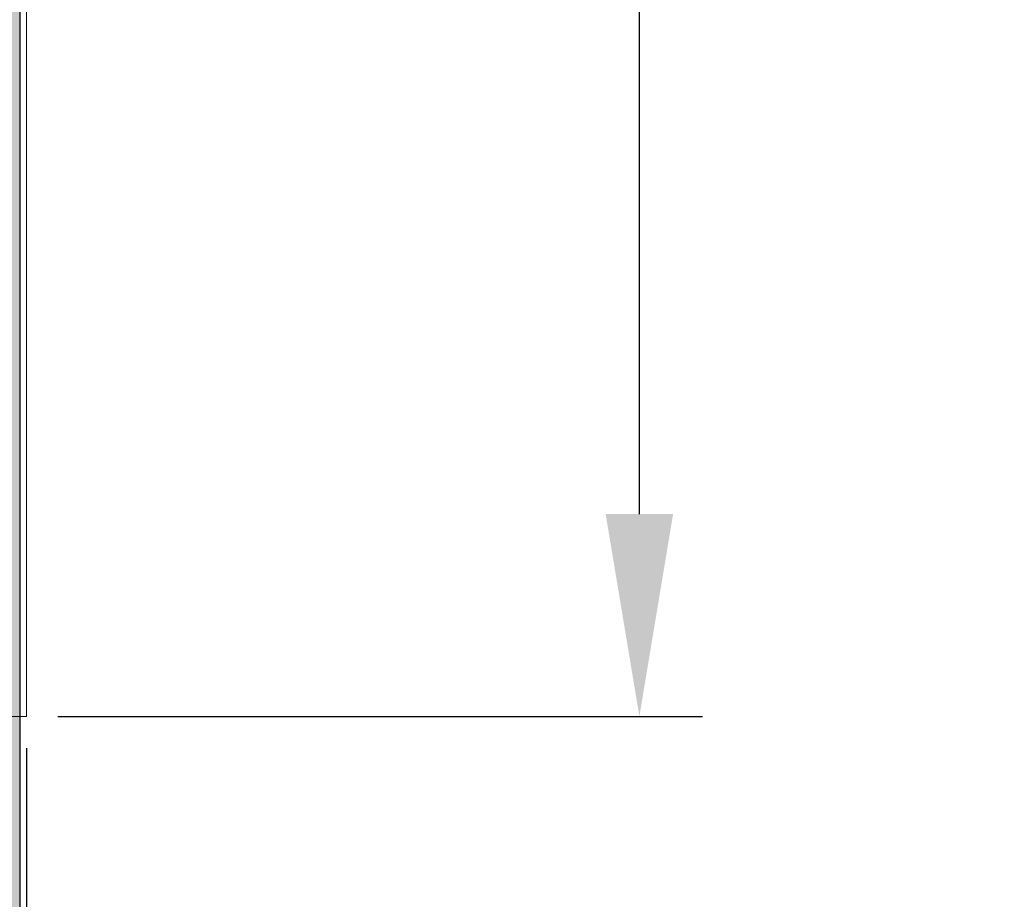
# Model space of a CAD drawing. Units: inches. Extents: x 2091 to 2899, y 967 to 2217.
# Tile 253 of 256: x 2212 to 2232, y 1149 to 1166. Entities that reach past the tile are written whole.
import ezdxf

# ---------------------------------------------------------------- set-up
doc = ezdxf.new("R2010")
doc.units = ezdxf.units.IN
doc.layers.add('A-ANNO-DIMS', color=2, linetype='Continuous', lineweight=18)
doc.layers.add('A-GLAZ', color=4, linetype='Continuous', lineweight=18)
doc.layers.add('A-WALL-PATT', color=141, linetype='Continuous', lineweight=13, true_color=0xadddf7)
doc.styles.get("Standard").update_dxf_attribs({"font": 'arial.ttf'})
doc.dimstyles.new('ISO-25', dxfattribs={"dimtxt": 4, "dimasz": 4, "dimexe": 1.25, "dimexo": 0.625, "dimtad": 1, "dimdec": 0, "dimlunit": 3, "dimtxsty": 'Standard', "dimcen": 2.5, "dimadec": 0, "dimazin": 0, "dimtfac": 1, "dimtdec": 0, "dimtmove": 0, "dimatfit": 3, "dimfxl": 1, "dimarcsym": 0})

# ---------------------------------------------------------------- blocks, each defined once
blk = doc.blocks.new('WIN-DOUBLE-LINE')
for p, q in [((9.16, 80.823), (9.16, 0)), ((9.16, 0), (0, 0))]:
    blk.add_line(p, q)
blk = doc.blocks.new('*D36')
at = {"layer": 'A-ANNO-DIMS', "color": 0, "lineweight": -2, "transparency": 16777216}
for p, q in [((2212.901, 1233.07), (2225.649, 1233.07)), ((2224.399, 1156.247), (2224.399, 1229.07)), ((2212.901, 1152.247), (2225.649, 1152.247))]:
    blk.add_line(p, q, dxfattribs=at)
at = {"layer": 'A-ANNO-DIMS', "color": 0, "transparency": 16777216}
for points in [[(2223.732, 1229.07), (2225.066, 1229.07), (2224.399, 1233.07)], [(2223.732, 1156.247), (2225.066, 1156.247), (2224.399, 1152.247)]]:
    blk.add_solid(points, dxfattribs=at)
at = {"layer": 'Defpoints', "color": 0, "transparency": 16777216}
for p in [(2212.276, 1233.07), (2224.399, 1233.07), (2212.276, 1152.247)]:
    blk.add_point(p, dxfattribs=at)
at = {"layer": 'A-ANNO-DIMS', "color": 0, "transparency": 16777216, "insert": (2221.705, 1192.659), "char_height": 4, "attachment_point": 5, "rotation": 90}
blk.add_mtext('WINDOW 6\'-9" TYP.', dxfattribs=at)
blk = doc.blocks.new('*D37')
at = {"layer": 'A-ANNO-DIMS', "color": 0, "lineweight": -2, "transparency": 16777216}
for p, q in [((2203.116, 1151.622), (2203.116, 1138.874)), ((2212.276, 1151.622), (2212.276, 1138.874)), ((2199.116, 1140.124), (2195.116, 1140.124)), ((2203.116, 1140.124), (2212.276, 1140.124)), ((2216.276, 1140.124), (2245.908, 1140.124))]:
    blk.add_line(p, q, dxfattribs=at)
at = {"layer": 'A-ANNO-DIMS', "color": 0, "transparency": 16777216}
for points in [[(2199.116, 1140.79), (2199.116, 1139.457), (2203.116, 1140.124)], [(2216.276, 1140.79), (2216.276, 1139.457), (2212.276, 1140.124)]]:
    blk.add_solid(points, dxfattribs=at)
at = {"layer": 'Defpoints', "color": 0, "transparency": 16777216}
for p in [(2203.116, 1152.247), (2212.276, 1152.247), (2212.276, 1140.124)]:
    blk.add_point(p, dxfattribs=at)
at = {"layer": 'A-ANNO-DIMS', "color": 0, "transparency": 16777216, "insert": (2233.092, 1142.791), "char_height": 4, "attachment_point": 5}
blk.add_mtext('0\'-9" TYP.', dxfattribs=at)
blk = doc.blocks.new('*D71')
at = {"layer": 'A-ANNO-DIMS', "color": 0, "lineweight": -2, "transparency": 16777216}
for p, q in [((2212.144, 1351.294), (2212.144, 969.464)), ((2452.144, 1351.294), (2452.144, 969.464)), ((2216.144, 970.714), (2448.144, 970.714))]:
    blk.add_line(p, q, dxfattribs=at)
at = {"layer": 'A-ANNO-DIMS', "color": 0, "transparency": 16777216}
for points in [[(2216.144, 971.381), (2216.144, 970.048), (2212.144, 970.714)], [(2448.144, 971.381), (2448.144, 970.048), (2452.144, 970.714)]]:
    blk.add_solid(points, dxfattribs=at)
at = {"layer": 'Defpoints', "color": 0, "transparency": 16777216}
for p in [(2212.144, 1351.919), (2452.144, 1351.919), (2452.144, 970.714)]:
    blk.add_point(p, dxfattribs=at)
at = {"layer": 'A-ANNO-DIMS', "color": 0, "transparency": 16777216, "insert": (2332.144, 973.382), "char_height": 4, "attachment_point": 5}
blk.add_mtext('20\'-0"', dxfattribs=at)
blk = doc.blocks.new('*D75')
at = {"layer": 'A-ANNO-DIMS', "color": 0, "lineweight": -2, "transparency": 16777216}
for p, q in [((2212.144, 1274.794), (2212.144, 969.464)), ((2308.144, 1274.794), (2308.144, 969.464)), ((2216.144, 970.714), (2304.144, 970.714))]:
    blk.add_line(p, q, dxfattribs=at)
at = {"layer": 'A-ANNO-DIMS', "color": 0, "transparency": 16777216}
for points in [[(2216.144, 971.381), (2216.144, 970.048), (2212.144, 970.714)], [(2304.144, 971.381), (2304.144, 970.048), (2308.144, 970.714)]]:
    blk.add_solid(points, dxfattribs=at)
at = {"layer": 'Defpoints', "color": 0, "transparency": 16777216}
for p in [(2212.144, 1275.419), (2308.144, 1275.419), (2308.144, 970.714)]:
    blk.add_point(p, dxfattribs=at)
at = {"layer": 'A-ANNO-DIMS', "color": 0, "transparency": 16777216, "insert": (2260.144, 973.382), "char_height": 4, "attachment_point": 5}
blk.add_mtext('8\'-0"', dxfattribs=at)
blk = doc.blocks.new('*D91')
at = {"layer": 'A-ANNO-DIMS', "color": 0, "lineweight": -2, "transparency": 16777216}
for p, q in [((2211.651, 1152.247), (2098.311, 1152.247)), ((2099.561, 1103.919), (2099.561, 1148.247)), ((2211.519, 1099.919), (2098.311, 1099.919))]:
    blk.add_line(p, q, dxfattribs=at)
at = {"layer": 'A-ANNO-DIMS', "color": 0, "transparency": 16777216}
for points in [[(2098.895, 1148.247), (2100.228, 1148.247), (2099.561, 1152.247)], [(2098.895, 1103.919), (2100.228, 1103.919), (2099.561, 1099.919)]]:
    blk.add_solid(points, dxfattribs=at)
at = {"layer": 'Defpoints', "color": 0, "transparency": 16777216}
for p in [(2099.561, 1152.247), (2212.276, 1152.247), (2212.144, 1099.919)]:
    blk.add_point(p, dxfattribs=at)
at = {"layer": 'A-ANNO-DIMS', "color": 0, "transparency": 16777216, "insert": (2096.868, 1126.083), "char_height": 4, "attachment_point": 5, "rotation": 90}
blk.add_mtext('4\'-4 1/2"', dxfattribs=at)

msp = doc.modelspace()

# ---------------------------------------------------------------- hatches: boundary and pattern name
at = {"layer": 'A-WALL-PATT'}
h = msp.add_hatch(color=256, dxfattribs=at)
h.dxf.hatch_style = 1
h.paths.add_polyline_path([(2803.144, 2050.919), (2203.144, 2050.919), (2203.144, 1090.919), (2803.144, 1090.919)])
h.paths.add_polyline_path([(2635.799, 1147.54), (2674.524, 1147.54, 0.376086), (2678.53, 1152.88), (2678.53, 1159.556, 0.333335), (2674.524, 1163.562), (2674.524, 1163.562), (2674.524, 1192.934), (2635.806, 1192.934), (2597.088, 1192.934), (2597.088, 1163.562, 0.333335), (2593.082, 1159.556), (2593.082, 1152.88, 0.376086), (2597.088, 1147.54)], flags=0)
h.paths.add_polyline_path([(2436.01, 1278.241, 0.000483), (2435.953, 1278.215, -0.001328), (2435.936, 1278.112, -0.001711), (2436.116, 1278.041, 0.002185)], flags=0)
h.paths.add_polyline_path([(2794.144, 1143.419), (2794.144, 1347.419), (2543.37, 1347.419), (2543.37, 1351.919), (2794.144, 1351.919), (2794.144, 1392.714), (2793.947, 1392.714), (2793.947, 1473.537), (2794.144, 1473.537), (2794.144, 1531.919), (2650.144, 1531.919), (2650.144, 1536.419), (2794.144, 1536.419), (2794.144, 1692.419), (2609.376, 1692.419), (2609.376, 1644.419), (2604.876, 1644.419), (2604.876, 1744.919), (2609.376, 1744.919), (2609.376, 1696.919), (2794.144, 1696.919), (2794.144, 1780.919), (2609.644, 1780.919), (2493.876, 1780.919), (2493.876, 1785.419), (2609.644, 1785.419), (2794.144, 1785.419), (2794.144, 1847.939), (2793.951, 1847.939), (2793.951, 1928.762), (2794.144, 1928.762), (2794.144, 1941.419), (2614.144, 1941.419), (2614.144, 1821.419), (2609.644, 1821.419), (2609.644, 1941.419), (2392.144, 1941.419), (2392.144, 1819.919), (2387.644, 1819.919), (2387.644, 1941.419), (2212.144, 1941.419), (2212.144, 1783.919), (2392.144, 1783.919), (2392.144, 1780.919), (2212.144, 1780.919), (2212.144, 1629.419), (2387.644, 1629.419), (2387.644, 1744.919), (2392.144, 1744.919), (2392.144, 1627.919), (2317.144, 1627.919), (2317.144, 1551.419), (2317.144, 1536.419), (2459.384, 1536.419), (2459.384, 1602.396), (2463.884, 1602.396), (2463.884, 1531.919), (2456.644, 1531.919), (2456.644, 1529.919), (2452.144, 1529.919), (2452.144, 1531.919), (2312.644, 1531.919), (2312.644, 1551.419), (2306.144, 1551.419), (2306.144, 1555.919), (2308.144, 1555.919), (2308.144, 1551.419), (2312.644, 1551.419), (2312.644, 1627.919), (2212.144, 1627.919), (2212.144, 1555.919), (2270.144, 1555.919), (2270.144, 1551.419), (2212.144, 1551.419), (2212.144, 1351.919), (2272.144, 1351.919), (2272.144, 1347.419), (2212.144, 1347.419), (2212.144, 1275.419), (2308.144, 1275.419), (2308.144, 1351.919), (2452.144, 1351.919), (2452.144, 1493.919), (2456.644, 1493.919), (2456.644, 1347.419), (2312.644, 1347.419), (2312.644, 1270.919), (2212.144, 1270.919), (2212.144, 1099.919), (2281.238, 1099.919), (2282.871, 1110.914), (2282.008, 1116.997), (2278.558, 1121.42), (2268.206, 1128.056), (2272.088, 1128.056), (2273.813, 1131.927), (2279.42, 1134.692), (2285.028, 1135.245), (2287.616, 1137.457), (2288.047, 1138.01), (2289.341, 1140.775), (2291.067, 1139.669), (2292.361, 1135.245), (2295.38, 1136.904), (2296.243, 1135.798), (2297.105, 1133.033), (2300.125, 1138.01), (2303.144, 1138.01), (2304.438, 1135.798), (2303.144, 1133.586), (2306.595, 1134.692), (2307.889, 1133.033), (2310.908, 1135.245), (2313.927, 1134.139), (2315.627, 1132.427), (2308.32, 1117.55), (2290.204, 1109.808), (2288.91, 1103.172), (2289.272, 1099.919), (2434.918, 1099.919), (2431.593, 1124.788), (2429.93, 1169.553), (2430.927, 1240.52), (2435.659, 1238.186), (2437.135, 1196.554), (2438.798, 1143.973), (2442.678, 1111.998), (2446.558, 1099.919), (2794.144, 1099.919), (2794.144, 1138.919), (2548.032, 1138.919), (2548.032, 1143.419), (2548.032, 1148.819), (2546.668, 1148.032), (2528.686, 1179.179, 0.256256), (2512.032, 1148.819), (2512.032, 1143.419), (2512.032, 1138.919), (2507.532, 1138.919), (2507.532, 1143.419), (2507.532, 1148.819, 0.256256), (2490.879, 1179.179), (2472.896, 1148.032), (2471.532, 1148.819), (2471.532, 1143.419), (2467.032, 1143.419), (2467.032, 1269.946, 0.039061), (2460.91, 1273.58), (2467.032, 1273.58), (2467.032, 1286.325, 0.014511), (2465.216, 1286.762), (2467.032, 1287.053), (2467.032, 1323.419), (2471.532, 1323.419), (2471.532, 1148.819), (2489.532, 1179.996), (2490.896, 1179.208), (2490.879, 1179.179, -0.256256), (2507.532, 1148.819), (2507.532, 1143.419), (2512.032, 1143.419), (2512.032, 1148.819, -0.256256), (2528.686, 1179.179), (2528.668, 1179.208), (2530.032, 1179.996), (2548.032, 1148.819), (2548.032, 1143.419)], flags=16)
h.paths.add_polyline_path([(2607.769, 1200.945), (2607.769, 1265.031), (2597.088, 1281.052), (2619.785, 1281.052), (2627.795, 1337.127), (2635.799, 1337.127), (2643.817, 1337.127), (2651.827, 1281.052), (2674.524, 1281.052), (2663.843, 1265.031), (2663.843, 1200.945), (2635.806, 1200.945)], flags=0)
edge = h.paths.add_edge_path(flags=0)
edge.add_ellipse((13303.896, 1272.999), major_axis=(-10595.313, 0), ratio=0.84230387, start_angle=0.6282372, end_angle=0.6465541, ccw=False)
edge.add_ellipse((2711.7, 1156.853), major_axis=(2.22, 0), ratio=0.842304, start_angle=111.5352, end_angle=180.6282, ccw=False)
edge.add_ellipse((13303.156, 1272.999), major_axis=(-10593.026, 0), ratio=0.84230387, start_angle=0.5282715, end_angle=0.6465541, ccw=False)
edge.add_line((2710.765, 1175.333), (2710.13, 1175.333))
edge.add_ellipse((2710.13, 1176.58), major_axis=(1.48, 0), ratio=0.842304, start_angle=180, end_angle=270, ccw=False)
edge.add_line((2708.65, 1176.58), (2708.65, 1200.783))
edge.add_ellipse((2710.13, 1200.783), major_axis=(1.48, 0), ratio=0.842304, start_angle=90, end_angle=180, ccw=False)
edge.add_line((2710.13, 1202.029), (2710.465, 1202.029))
edge.add_ellipse((13303.156, 1272.999), major_axis=(-10593.026, 0), ratio=0.84230387, start_angle=-0.0902291, end_angle=0.3838668, ccw=False)
edge.add_ellipse((2710.13, 1290.927), major_axis=(-1.48, 0), ratio=0.842304, start_angle=0, end_angle=90, ccw=False)
edge.add_line((2708.65, 1290.927), (2708.65, 1315.13))
edge.add_ellipse((2710.13, 1315.13), major_axis=(-1.48, 0), ratio=0.842304, start_angle=-90, end_angle=0, ccw=False)
edge.add_line((2710.13, 1316.377), (2710.706, 1316.377))
edge.add_ellipse((3238.402, 1296.29), major_axis=(528.234, 0), ratio=0.8423039, start_angle=176.34957, end_angle=177.82005, ccw=False)
edge.add_ellipse((2775.063, 1071.451), major_axis=(313.308, 0), ratio=0.8423039, start_angle=102.12597, end_angle=103.78053, ccw=False)
edge.add_ellipse((2775.063, 1078.306), major_axis=(-305.303, 0), ratio=0.8423039, start_angle=-79.79046, end_angle=-77.55537, ccw=False)
edge.add_ellipse((2695.142, 1541.975), major_axis=(-250.96, 0), ratio=0.8423039, start_angle=99.25657, end_angle=102.55493)
edge.add_line((2741.41, 1334.214), (2747.133, 1337.378))
edge.add_ellipse((2747.539, 1336.857), major_axis=(-0.74, 0), ratio=0.842304, start_angle=270, end_angle=307.9331, ccw=False)
edge.add_ellipse((2747.539, 1336.857), major_axis=(-0.74, 0), ratio=0.842304, start_angle=232.0669, end_angle=270, ccw=False)
edge.add_line((2747.945, 1337.378), (2753.667, 1334.214))
edge.add_ellipse((2799.935, 1541.975), major_axis=(250.96, 0), ratio=0.8423039, start_angle=257.44507, end_angle=260.74343)
edge.add_ellipse((2720.014, 1078.306), major_axis=(305.303, 0), ratio=0.8423039, start_angle=77.55537, end_angle=79.79046, ccw=False)
edge.add_ellipse((2720.014, 1071.451), major_axis=(-313.308, 0), ratio=0.8423039, start_angle=256.21947, end_angle=257.87403, ccw=False)
edge.add_ellipse((2256.676, 1296.29), major_axis=(-528.234, 0), ratio=0.8423039, start_angle=182.17995, end_angle=183.65043, ccw=False)
edge.add_line((2784.371, 1316.377), (2784.947, 1316.377))
edge.add_ellipse((2784.947, 1315.13), major_axis=(1.48, 0), ratio=0.842304, start_angle=0, end_angle=90, ccw=False)
edge.add_line((2786.427, 1315.13), (2786.427, 1290.927))
edge.add_ellipse((2784.947, 1290.927), major_axis=(1.48, 0), ratio=0.842304, start_angle=270, end_angle=360, ccw=False)
edge.add_ellipse((-7808.079, 1272.999), major_axis=(10593.026, 0), ratio=0.84230387, start_angle=-0.3838668, end_angle=0.0902291, ccw=False)
edge.add_line((2784.612, 1202.029), (2784.947, 1202.029))
edge.add_ellipse((2784.947, 1200.783), major_axis=(1.48, 0), ratio=0.842304, start_angle=0, end_angle=90, ccw=False)
edge.add_line((2786.427, 1200.783), (2786.427, 1176.58))
edge.add_ellipse((2784.947, 1176.58), major_axis=(-1.48, 0), ratio=0.842304, start_angle=90, end_angle=180, ccw=False)
edge.add_line((2784.947, 1175.333), (2784.313, 1175.333))
edge.add_ellipse((-7808.079, 1272.999), major_axis=(10593.026, 0), ratio=0.84230387, start_angle=-0.6186432, end_angle=-0.5282715, ccw=False)
edge.add_ellipse((2783.377, 1156.853), major_axis=(-2.22, 0), ratio=0.842304, start_angle=179.3718, end_angle=248.4648, ccw=False)
edge.add_ellipse((-7808.819, 1272.999), major_axis=(-10595.313, 0), ratio=0.842303866, start_angle=179.3534459, end_angle=179.3717628, ccw=False)
edge.add_ellipse((2780.297, 1153.501), major_axis=(-5.246, 0), ratio=0.842304, start_angle=90, end_angle=179.3534, ccw=False)
edge.add_line((2780.297, 1149.082), (2714.78, 1149.082))
edge.add_ellipse((2714.78, 1153.501), major_axis=(5.246, 0), ratio=0.842304, start_angle=180.6466, end_angle=270, ccw=False)
edge = h.paths.add_edge_path(flags=0)
edge.add_line((2718.187, 1151.008), (2718.187, 1170.472))
edge.add_ellipse((2721.147, 1170.472), major_axis=(-2.96, 0), ratio=0.842304, start_angle=-90, end_angle=0, ccw=False)
edge.add_line((2721.147, 1172.965), (2773.93, 1172.965))
edge.add_ellipse((2773.93, 1170.472), major_axis=(-2.96, 0), ratio=0.842304, start_angle=180, end_angle=270, ccw=False)
edge.add_line((2776.89, 1170.472), (2776.89, 1151.008))
edge.add_line((2776.89, 1151.008), (2718.187, 1151.008))
edge = h.paths.add_edge_path(flags=0)
edge.add_line((2718.187, 1180.234), (2718.187, 1199.058))
edge.add_ellipse((2747.539, 1320.399), major_axis=(147.018, 0), ratio=0.8423039, start_angle=256.40187, end_angle=283.59813)
edge.add_line((2776.89, 1199.058), (2776.89, 1180.234))
edge.add_ellipse((2747.539, 1301.575), major_axis=(147.018, 0), ratio=0.8423039, start_angle=256.40187, end_angle=283.59813, ccw=False)
edge = h.paths.add_edge_path(flags=0)
edge.add_ellipse((13303.156, 1272.999), major_axis=(-10591.546, 0), ratio=0.84230387, start_angle=0.0555943, end_angle=0.3777642, ccw=False)
edge.add_line((2711.617, 1262.722), (2715.667, 1249.495))
edge.add_ellipse((6413.892, 1241.692), major_axis=(-3698.236, 0), ratio=0.84230387, start_angle=-0.120897, end_angle=0.364076)
edge.add_line((2715.761, 1218.192), (2711.934, 1203.167))
edge = h.paths.add_edge_path(flags=0)
edge.add_line((2718.187, 1251.075), (2716.002, 1267.45))
edge.add_ellipse((2742.151, 1202.19), major_axis=(81.773, 0), ratio=0.842304, start_angle=94.27742, end_angle=111.83495, ccw=False)
edge.add_line((2737.01, 1270.931), (2758.067, 1270.931))
edge.add_ellipse((2752.926, 1202.19), major_axis=(81.773, 0), ratio=0.842304, start_angle=68.16505, end_angle=85.72258, ccw=False)
edge.add_line((2779.075, 1267.45), (2776.89, 1251.075))
edge.add_ellipse((2750.338, 1187.885), major_axis=(79.58, 0), ratio=0.842304, start_angle=67.20809, end_angle=85.12993)
edge.add_line((2756.035, 1254.744), (2739.043, 1254.744))
edge.add_ellipse((2744.739, 1187.885), major_axis=(79.58, 0), ratio=0.842304, start_angle=94.87007, end_angle=112.79191)
edge = h.paths.add_edge_path(flags=0)
edge.add_line((2783.143, 1203.167), (2779.316, 1218.192))
edge.add_ellipse((-918.815, 1241.692), major_axis=(3698.236, 0), ratio=0.84230387, start_angle=-0.364076, end_angle=0.120897)
edge.add_line((2779.41, 1249.495), (2783.46, 1262.722))
edge.add_ellipse((-7808.079, 1272.999), major_axis=(-10591.546, 0), ratio=0.84230387, start_angle=179.6222358, end_angle=179.9444057, ccw=False)
edge = h.paths.add_edge_path(flags=0)
edge.add_ellipse((2734.201, 1286.69), major_axis=(-0.357, 6.34), ratio=0.603834, start_angle=89.002, end_angle=253.6574, ccw=False)
edge.add_line((2730.369, 1286.542), (2730.369, 1301.352))
edge.add_line((2730.369, 1301.352), (2735.913, 1305.215))
edge.add_ellipse((2736.385, 1304.735), major_axis=(0.74, 0), ratio=0.842304, start_angle=90, end_angle=134.4802, ccw=False)
edge.add_line((2736.385, 1305.358), (2738.033, 1305.358))
edge.add_line((2738.033, 1305.358), (2738.033, 1307.708))
edge.add_ellipse((2794.202, 1307.708), major_axis=(56.169, 0), ratio=0.842304, start_angle=150.5614, end_angle=180, ccw=False)
edge.add_ellipse((2700.876, 1307.708), major_axis=(-56.169, 0), ratio=0.842304, start_angle=180, end_angle=209.4386, ccw=False)
edge.add_line((2757.044, 1307.708), (2757.044, 1305.358))
edge.add_line((2757.044, 1305.358), (2758.692, 1305.358))
edge.add_ellipse((2758.692, 1304.735), major_axis=(-0.74, 0), ratio=0.842304, start_angle=225.5198, end_angle=270, ccw=False)
edge.add_line((2759.164, 1305.215), (2764.708, 1301.352))
edge.add_line((2764.708, 1301.352), (2764.708, 1286.542))
edge.add_ellipse((2760.876, 1286.69), major_axis=(0.357, 6.34), ratio=0.603834, start_angle=106.3426, end_angle=270.998, ccw=False)
edge.add_line((2757.044, 1285.797), (2757.044, 1307.708))
edge.add_ellipse((2700.876, 1307.708), major_axis=(-56.169, 0), ratio=0.842304, start_angle=180, end_angle=209.4386)
edge.add_ellipse((2794.202, 1307.708), major_axis=(56.169, 0), ratio=0.842304, start_angle=150.5614, end_angle=180)
edge.add_line((2738.033, 1307.708), (2738.033, 1285.797))
h.paths.add_polyline_path([(2417.812, 1104.45), (2413.492, 1102.53), (2410.612, 1103.97), (2409.172, 1106.37), (2407.252, 1107.33), (2406.292, 1109.73), (2405.332, 1114.05), (2405.332, 1117.89), (2406.292, 1120.13), (2407.252, 1119.81), (2408.848, 1118.328), (2410.174, 1119.424), (2410.211, 1120.406), (2411.041, 1121.419), (2410.699, 1119.859), (2410.174, 1119.424), (2410.088, 1117.176), (2411.133, 1116.206), (2413.972, 1119.33), (2416.852, 1120.77), (2416.87, 1120.799), (2417.035, 1119.405), (2417.896, 1118.143), (2418.292, 1118.37), (2419.544, 1120.039), (2419.361, 1118.387), (2419.032, 1119.356), (2418.399, 1118.512), (2419.252, 1114.53), (2418.794, 1107.199)], flags=0)
h.paths.add_polyline_path([(2508.87, 1347.419), (2508.37, 1347.419), (2508.37, 1351.919), (2508.87, 1351.919)], flags=0)
h.paths.add_polyline_path([(2473.37, 1347.419), (2472.37, 1347.419), (2467.87, 1347.419), (2467.87, 1455.419), (2472.37, 1455.419), (2472.37, 1352.419), (2473.37, 1352.419)], flags=0)
h.paths.add_polyline_path([(2352.106, 1217.446), (2349.226, 1218.886), (2347.786, 1221.286), (2345.866, 1222.246), (2344.906, 1224.646), (2343.946, 1228.966), (2343.946, 1232.806), (2344.906, 1235.046), (2345.866, 1234.726), (2347.462, 1233.244), (2348.788, 1234.341), (2348.825, 1235.322), (2349.655, 1236.336), (2349.313, 1234.775), (2348.788, 1234.341), (2348.702, 1232.093), (2349.747, 1231.123), (2352.586, 1234.246), (2355.466, 1235.686), (2355.484, 1235.715), (2355.649, 1234.322), (2356.51, 1233.06), (2356.906, 1233.286), (2358.158, 1234.956), (2357.975, 1233.304), (2357.646, 1234.273), (2357.013, 1233.428), (2357.866, 1229.446), (2357.408, 1222.115), (2356.426, 1219.366)], flags=0)
h.paths.add_polyline_path([(2348.297, 1112.224), (2347.014, 1112.31), (2345.53, 1114.127), (2345.732, 1115.858), (2346.812, 1116.982), (2346.812, 1114.646), (2345.867, 1114.214), (2346.88, 1114.3)], flags=0)
h.paths.add_polyline_path([(2347.014, 1110.926), (2346.272, 1110.493), (2346.61, 1111.186)], flags=0)
h.paths.add_polyline_path([(2345.867, 1118.194), (2345.53, 1117.329), (2343.708, 1118.021), (2344.383, 1118.626)], flags=0)
h.paths.add_polyline_path([(2346.677, 1109.282), (2346.07, 1108.071), (2345.867, 1110.061)], flags=0)
h.paths.add_polyline_path([(2345.057, 1119.751), (2343.64, 1119.751), (2343.978, 1121.135)], flags=0)
h.paths.add_polyline_path([(2345.26, 1116.55), (2345.125, 1115.858), (2344.922, 1115.685), (2344.72, 1116.377)], flags=0)
h.paths.add_polyline_path([(2345.665, 1112.31), (2345.462, 1111.532), (2344.045, 1111.964), (2344.652, 1112.57)], flags=0)
h.paths.add_polyline_path([(2345.192, 1113.349), (2344.45, 1113.868), (2344.72, 1114.387)], flags=0)
h.paths.add_polyline_path([(2344.652, 1116.809), (2344.18, 1115.685), (2344.652, 1115.339), (2343.91, 1114.906), (2343.033, 1115.944), (2343.64, 1116.463)], flags=0)
h.paths.add_polyline_path([(2345.867, 1106.686), (2344.99, 1105.562), (2344.517, 1106.6)], flags=0)
h.paths.add_polyline_path([(2344.855, 1110.061), (2344.517, 1109.282), (2344.113, 1109.715)], flags=0)
h.paths.add_polyline_path([(2344.045, 1113.522), (2343.438, 1113.089), (2342.763, 1113.954)], flags=0)
h.paths.add_polyline_path([(2344.315, 1111.012), (2342.965, 1110.32), (2342.965, 1111.099)], flags=0)
h.paths.add_polyline_path([(2345.125, 1104.697), (2344.585, 1103.745), (2344.45, 1104.264)], flags=0)
h.paths.add_polyline_path([(2342.83, 1121.222), (2341.75, 1120.53), (2340.536, 1121.049), (2340.131, 1121.828), (2340.671, 1122.952), (2341.143, 1121.828), (2341.615, 1122.001)], flags=0)
h.paths.add_polyline_path([(2342.965, 1119.751), (2343.033, 1118.453), (2342.088, 1118.021), (2342.02, 1119.491)], flags=0)
h.paths.add_polyline_path([(2342.695, 1116.896), (2341.953, 1116.636), (2342.02, 1117.329)], flags=0)
h.paths.add_polyline_path([(2343.033, 1112.224), (2342.02, 1111.791), (2341.548, 1112.224), (2342.358, 1113.349)], flags=0)
h.paths.add_polyline_path([(2343.775, 1104.437), (2342.628, 1102.88), (2342.695, 1104.61), (2343.438, 1105.129)], flags=0)
h.paths.add_polyline_path([(2342.02, 1115.079), (2340.806, 1115.512), (2340.941, 1116.377)], flags=0)
h.paths.add_polyline_path([(2341.481, 1120.097), (2341.481, 1119.405), (2341.076, 1119.578), (2341.143, 1120.097)], flags=0)
h.paths.add_polyline_path([(2341.818, 1114.473), (2340.941, 1113.089), (2340.806, 1114.56)], flags=0)
h.paths.add_polyline_path([(2341.143, 1118.54), (2340.941, 1116.982), (2339.051, 1117.675), (2339.051, 1118.626)], flags=0)
h.paths.add_polyline_path([(2342.695, 1101.668), (2341.953, 1101.841), (2342.56, 1102.361)], flags=0)
h.paths.add_polyline_path([(2340.333, 1119.665), (2338.444, 1119.578), (2337.904, 1120.357), (2339.658, 1120.616)], flags=0)
h.paths.add_polyline_path([(2340.333, 1115.339), (2340.063, 1113.695), (2339.388, 1115.339)], flags=0)
h.paths.add_polyline_path([(2341.818, 1103.831), (2341.548, 1102.88), (2341.143, 1103.658)], flags=0)
h.paths.add_polyline_path([(2339.051, 1122.866), (2337.296, 1121.828), (2337.094, 1123.125), (2337.769, 1123.818)], flags=0)
h.paths.add_polyline_path([(2339.118, 1121.741), (2338.848, 1121.222), (2338.174, 1121.049), (2338.376, 1121.568)], flags=0)
h.paths.add_polyline_path([(2339.186, 1119.319), (2338.646, 1118.713), (2338.241, 1118.107), (2338.241, 1118.886)], flags=0)
h.paths.add_polyline_path([(2341.143, 1101.928), (2340.603, 1101.236), (2340.063, 1101.841), (2340.603, 1102.361)], flags=0)
h.paths.add_polyline_path([(2337.634, 1117.761), (2336.621, 1118.28), (2337.296, 1118.972)], flags=0)
h.paths.add_polyline_path([(2336.824, 1119.578), (2334.799, 1118.972), (2335.204, 1120.357), (2336.554, 1120.876)], flags=0)
h.paths.add_polyline_path([(2339.118, 1100.457), (2337.364, 1100.543), (2336.756, 1101.236)], flags=0)
h.paths.add_polyline_path([(2336.351, 1122.433), (2336.014, 1121.914), (2334.934, 1122.433), (2334.529, 1123.471), (2335.744, 1122.779)], flags=0)
h.paths.add_polyline_path([(2334.732, 1120.876), (2334.259, 1120.357), (2334.057, 1120.789), (2334.597, 1121.308)], flags=0)
h.paths.add_polyline_path([(2334.462, 1122.174), (2332.572, 1121.308), (2331.357, 1122.174), (2332.1, 1122.866)], flags=0)
h.paths.add_polyline_path([(2334.259, 1118.54), (2333.382, 1118.453), (2333.652, 1119.319)], flags=0)
h.paths.add_polyline_path([(2335.542, 1102.274), (2334.192, 1102.62), (2335.272, 1103.312)], flags=0)
h.paths.add_polyline_path([(2332.707, 1119.665), (2331.695, 1120.443), (2332.505, 1120.789)], flags=0)
h.paths.add_polyline_path([(2334.732, 1101.149), (2333.517, 1101.582), (2333.989, 1101.755)], flags=0)
h.paths.add_polyline_path([(2332.64, 1116.636), (2331.087, 1116.29), (2331.965, 1118.194)], flags=0)
h.paths.add_polyline_path([(2330.75, 1121.568), (2330.277, 1120.27), (2328.523, 1119.319), (2328.995, 1121.049)], flags=0)
h.paths.add_polyline_path([(2330.75, 1118.626), (2330.008, 1117.502), (2329.873, 1118.021)], flags=0)
h.paths.add_polyline_path([(2332.1, 1102.361), (2330.547, 1102.014), (2331.695, 1102.966)], flags=0)
h.paths.add_polyline_path([(2329.535, 1113.608), (2329.063, 1112.31), (2328.59, 1113.349)], flags=0)
h.paths.add_polyline_path([(2328.388, 1117.848), (2327.51, 1116.55), (2327.173, 1117.761)], flags=0)
h.paths.add_polyline_path([(2329.738, 1106.513), (2329.535, 1105.302), (2328.253, 1106.081)], flags=0)
h.paths.add_polyline_path([(2328.658, 1114.387), (2328.05, 1114.127), (2328.32, 1114.906)], flags=0)
h.paths.add_polyline_path([(2328.32, 1112.224), (2327.106, 1112.137), (2326.701, 1112.656)], flags=0)
h.paths.add_polyline_path([(2326.903, 1115.252), (2326.701, 1114.127), (2325.216, 1113.608), (2326.093, 1115.339)], flags=0)
h.paths.add_polyline_path([(2326.633, 1108.33), (2326.093, 1107.379), (2325.891, 1108.503), (2326.498, 1109.109)], flags=0)
h.paths.add_polyline_path([(2615.144, 1531.919), (2609.644, 1531.919), (2609.644, 1620.419), (2614.144, 1620.419), (2614.144, 1536.419), (2615.144, 1536.419)], flags=0)
h.paths.add_polyline_path([(2545.144, 1563.419), (2464.144, 1563.419), (2464.144, 1632.419), (2509.144, 1632.419), (2509.144, 1627.919), (2509.144, 1603.919), (2468.644, 1603.919), (2468.644, 1567.919), (2540.644, 1567.919), (2540.644, 1591.919), (2545.144, 1591.919)], flags=0)
h.paths.add_polyline_path([(2388.969, 1549.986), (2357.434, 1549.986), (2357.434, 1623.361), (2399.363, 1623.361), (2435.689, 1623.361), (2435.593, 1602.559), (2435.593, 1602.396), (2388.969, 1602.396)], flags=0)
h.paths.add_polyline_path([(2388.881, 1555.809), (2374.904, 1555.809), (2374.904, 1600.572), (2374.904, 1615.458), (2406.351, 1615.458), (2406.351, 1618.939), (2412.174, 1615.458), (2406.351, 1611.976), (2406.351, 1615.458), (2388.881, 1615.458)], flags=0)
h.paths.add_polyline_path([(2568.876, 1644.419), (2453.376, 1644.419), (2453.376, 1785.419), (2457.876, 1785.419), (2457.876, 1648.919), (2568.876, 1648.919)], flags=0)
h.paths.add_polyline_path([(2212.144, 1945.919), (2212.144, 2041.919), (2794.144, 2041.919), (2794.144, 1945.919)], flags=16)
h.paths.add_polyline_path([(2271.083, 1964.317), (2776.853, 1964.317), (2776.853, 2037.17), (2271.083, 2037.17)], flags=8)
h.paths.add_polyline_path([(2380.649, 1536.824), (2461.041, 1536.824), (2461.041, 1554.653), (2380.649, 1554.653)], flags=8)
h.paths.add_polyline_path([(2240.756, 1609.725), (2309.186, 1609.725), (2309.186, 1617.698), (2240.756, 1617.698)], flags=8)
h.paths.add_polyline_path([(2212.677, 1313.504), (2282.592, 1313.504), (2282.592, 1322.745), (2212.677, 1322.745)], flags=8)
h.paths.add_polyline_path([(2457.112, 1114.779), (2558.482, 1114.779), (2558.482, 1142.22), (2457.112, 1142.22)], flags=8)
h.paths.add_polyline_path([(2473.442, 1273.01), (2604.641, 1273.01), (2604.641, 1318.347), (2473.442, 1318.347)], flags=8)
h.paths.add_polyline_path([(2638.876, 1626.977), (2684.25, 1627.977), (2684.038, 1637.597), (2638.664, 1636.598)], flags=8)
h.paths.add_polyline_path([(2537.591, 1453.793), (2628.39, 1453.793), (2628.39, 1475.345), (2537.591, 1475.345)], flags=8)
h.paths.add_polyline_path([(2504.138, 1714.632), (2554.647, 1714.632), (2554.647, 1730.238), (2504.138, 1730.238)], flags=8)
h.paths.add_polyline_path([(2487.501, 1575.652), (2535.097, 1575.652), (2535.097, 1598.378), (2487.501, 1598.378)], flags=8)
h.paths.add_polyline_path([(2709.099, 1735.71), (2740.017, 1735.71), (2740.017, 1749.938), (2709.099, 1749.938)], flags=8)
h.paths.add_polyline_path([(2442.438, 1792.172), (2564.729, 1792.172), (2564.729, 1842), (2442.438, 1842)], flags=8)
h.paths.add_polyline_path([(2655.816, 1809.644), (2789.52, 1806.694), (2790.085, 1832.292), (2656.381, 1835.242)], flags=8)
h.paths.add_polyline_path([(2234.843, 1797.72), (2368.593, 1794.769), (2369.161, 1820.504), (2235.411, 1823.455)], flags=8)
h.paths.add_polyline_path([(2245.138, 1644.006), (2398.428, 1640.624), (2398.995, 1666.325), (2245.706, 1669.707)], flags=8)
h.paths.add_polyline_path([(2306.143, 1431.169), (2413.768, 1428.794), (2414.333, 1454.392), (2306.708, 1456.766)], flags=8)
h.paths.add_polyline_path([(2306.835, 1458.233), (2393.38, 1456.323), (2393.933, 1481.354), (2307.387, 1483.264)], flags=8)

# ---------------------------------------------------------------- block references
at = {"layer": 'A-GLAZ'}
msp.add_blockref('WIN-DOUBLE-LINE', (2203.115, 1152.248), dxfattribs=at)

# ---------------------------------------------------------------- dimensions: what is measured, and where the dimension line sits
at = {"layer": 'A-ANNO-DIMS'}
for base, p1, p2, picture, middle in [((2452.144, 970.714), (2212.144, 1351.919), (2452.144, 1351.919), '*D71', (2332.144, 973.382)), ((2308.144, 970.714), (2212.144, 1275.419), (2308.144, 1275.419), '*D75', (2260.144, 973.382))]:
    dim = msp.add_linear_dim(base=base, p1=p1, p2=p2, dimstyle='ISO-25', override={"dimdec": 1, "dimlfac": 1, "dimrnd": 0, "dimzin": 1, "dimdsep": 46, "dimlunit": 4, "dimfrac": 2}, dxfattribs=at)
    dim.commit()
    dim.dimension.update_dxf_attribs({"geometry": picture, "text_midpoint": middle})
dim = msp.add_linear_dim(base=(2224.399, 1233.07), p1=(2212.276, 1152.247), p2=(2212.276, 1233.07), angle=90, text='WINDOW <> TYP.', dimstyle='ISO-25', override={"dimdec": 1, "dimlfac": 1, "dimrnd": 0, "dimzin": 1, "dimdsep": 46, "dimlunit": 4, "dimfrac": 2}, dxfattribs=at)
dim.commit()
dim.dimension.update_dxf_attribs({"geometry": '*D36', "text_midpoint": (2221.705, 1192.659)})
dim = msp.add_linear_dim(base=(2099.561, 1152.247), p1=(2212.144, 1099.919), p2=(2212.276, 1152.247), angle=90, dimstyle='ISO-25', override={"dimdec": 1, "dimlfac": 1, "dimrnd": 0, "dimzin": 1, "dimdsep": 46, "dimlunit": 4, "dimfrac": 2}, dxfattribs=at)
dim.commit()
dim.dimension.update_dxf_attribs({"geometry": '*D91', "text_midpoint": (2096.868, 1126.083)})
dim = msp.add_linear_dim(base=(2212.276, 1140.124), p1=(2203.116, 1152.247), p2=(2212.276, 1152.247), text='<> TYP.', dimstyle='ISO-25', override={"dimdec": 1, "dimlfac": 1, "dimrnd": 0, "dimzin": 1, "dimdsep": 46, "dimlunit": 4, "dimfrac": 2}, dxfattribs=at)
dim.commit()
dim.dimension.update_dxf_attribs({"geometry": '*D37', "text_midpoint": (2233.092, 1142.791)})

doc.saveas('drawing.dxf')
